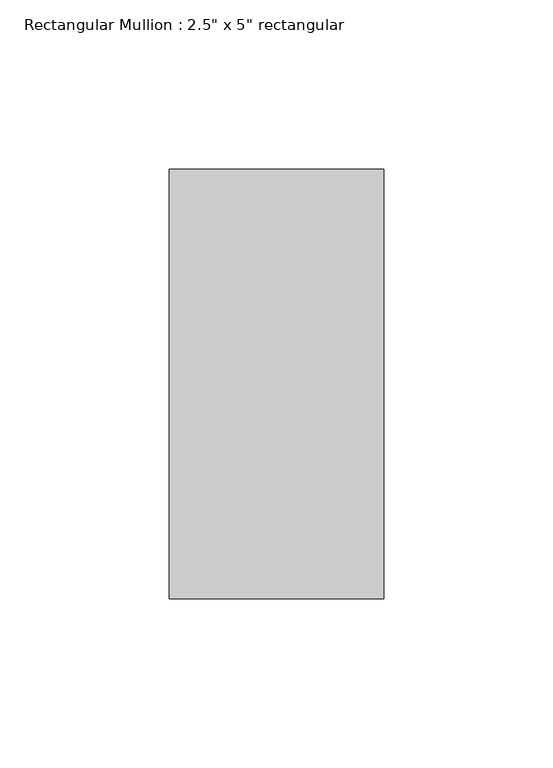
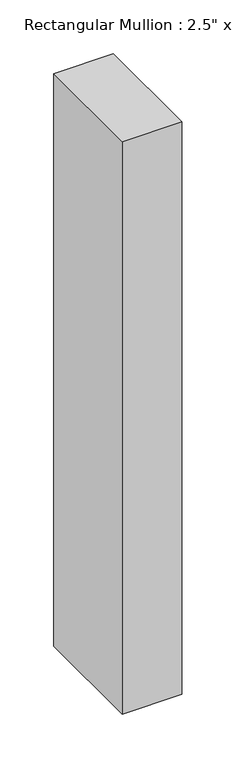
"""IFC4 building model written with IfcOpenShell, lengths in millimetres: member geometry."""

from ifc_helpers import new_model, si_unit, frame, origin, place, context, project, spatial, polyline, outline, extrude, source, transform, mapped, element, save


def member_8600bbed(model_context):
    return source(origin(), model_context, "Body", "SweptSolid", [
        extrude(outline(polyline([(0.0, 63.5), (0.0, -63.5), (-63.5, -63.5), (-63.5, 63.5), (0.0, 63.5)])), frame((0.0, 0.0, -648.4136426), z_axis=(0.0, 0.0, 1.0), x_axis=(1.0, 0.0, 0.0)), (0.0, 0.0, 1.0), 648.4136426),
    ])


if __name__ == "__main__":
    model = new_model("IFC4")
    model_context = context("Model", 3, world=origin())
    ifc_project = project(units=[si_unit("LENGTHUNIT", "METRE", prefix="MILLI")], contexts=[model_context])
    site = spatial("IfcSite", under=ifc_project)
    building = spatial("IfcBuilding", under=site)
    placement = place(None, origin())
    member_shape = member_8600bbed(model_context)
    element("IfcMember", 1, ObjectType="Rectangular Mullion : 2.5\" x 5\" rectangular", at=placement, inside=building, context=model_context, shape_type="MappedRepresentation", body=[
        mapped(member_shape, transform((0.0, 0.0, 0.0), x_axis=(1.0, 0.0, 0.0), y_axis=(0.0, 1.0, 0.0), z_axis=(0.0, 0.0, 1.0))),
    ])
    save(model, "model.ifc")

# Revit data of these elements
# Type "Rectangular Mullion : 2.5\" x 5\" rectangular"
#   built-in parameter 1007304 = 0.416667 (stored number, unit not read)
#   built-in parameter 1007301 = 0.104167 (stored number, unit not read)
#   built-in parameter 1007300 = 0.104167 (stored number, unit not read)
# Element 1 (IfcMember, "Rectangular Mullion : 2.5\" x 5\" rectangular")
#   Materials on its faces: "Aluminum"
# Materials
#   "Aluminum": class "Metal", colour RGB 247 247 247, transparency 0, Description = "Aluminum 6061", Cost = 0
